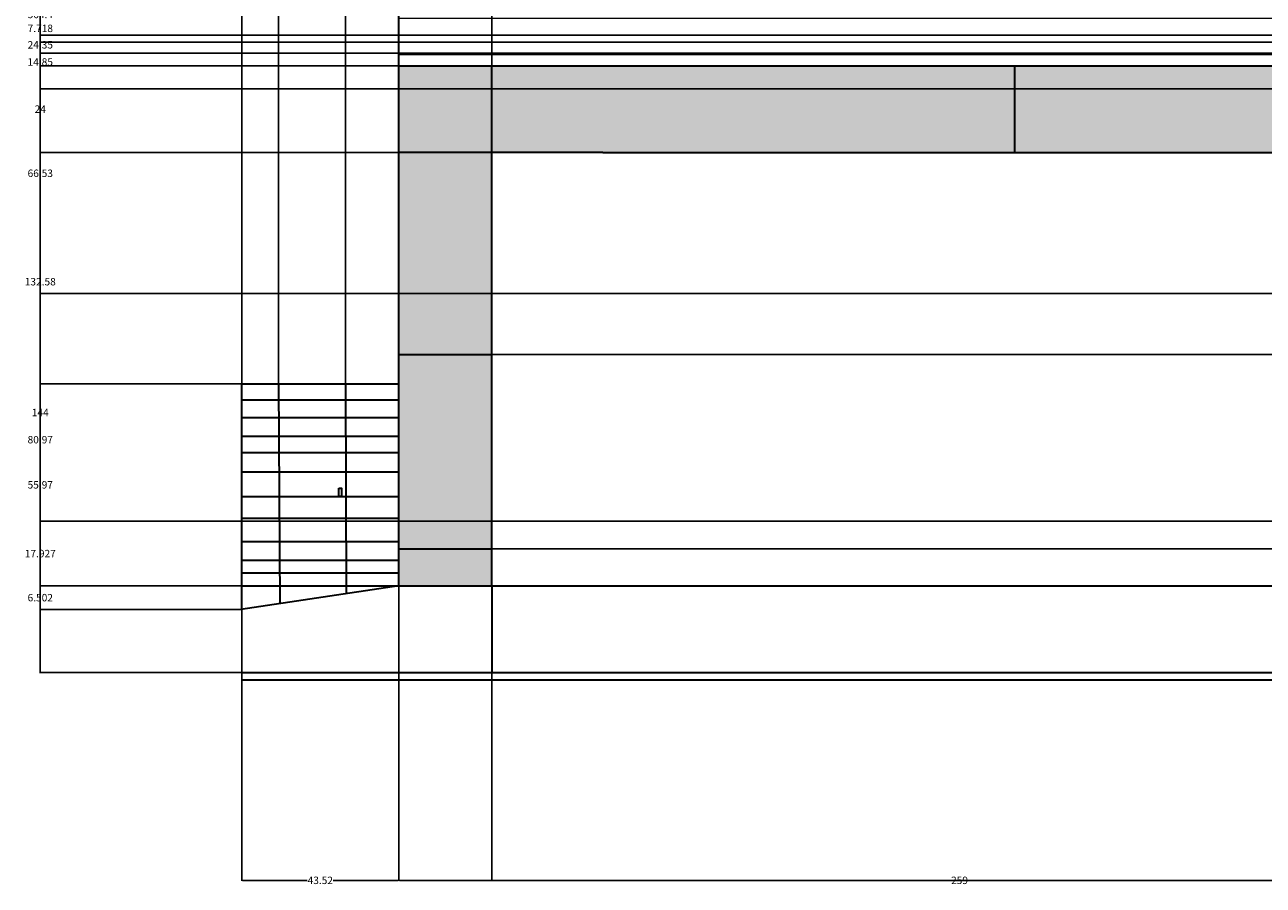
# Model space of a CAD drawing. Units: inches. Extents: x -30 to 1188, y 40 to 520.
# Tile 1 of 7: x -30 to 313, y 40 to 278. Entities that reach past the tile are written whole.
import ezdxf

# ---------------------------------------------------------------- set-up
doc = ezdxf.new("R2010")
doc.units = ezdxf.units.IN
doc.header["$MEASUREMENT"] = 0
for name, color, linetype, lineweight in [('A-ANNO-DIMS', 2, 'Continuous', 18), ('A-ELEV', 7, 'Continuous', 35), ('A-ELEV-PATT', 8, 'Continuous', 13)]:
    doc.layers.add(name, color=color, linetype=linetype, lineweight=lineweight)
doc.styles.get("Standard").update_dxf_attribs({"font": 'arial.ttf'})
doc.dimstyles.get("Standard").update_dxf_attribs({"dimtxt": 2.0625, "dimasz": 0.18, "dimexe": 0.18, "dimexo": 0.0625, "dimgap": 0.09, "dimtad": 0, "dimtih": 1, "dimtoh": 1, "dimdec": 4, "dimzin": 0, "dimdsep": 46, "dimlunit": 4, "dimtxsty": 'Standard', "dimcen": 0.09, "dimadec": 0, "dimazin": 0, "dimtfac": 1, "dimtdec": 4, "dimtofl": 0, "dimtmove": 0, "dimatfit": 3, "dimfxl": 1, "dimtolj": 1, "dimtzin": 0, "dimarcsym": 0})

# ---------------------------------------------------------------- blocks, each defined once
blk = doc.blocks.new('*D4')
at = {"layer": 'A-ANNO-DIMS', "color": 0, "lineweight": -2, "transparency": 16777216}
for p, q in [((73.66, 122.81), (73.66, 41.19)), ((1107.88, 118.31), (1107.88, 41.19)), ((73.84, 41.37), (586.5, 41.37)), ((1107.7, 41.37), (595.03, 41.37))]:
    blk.add_line(p, q, dxfattribs=at)
at = {"layer": 'A-ANNO-DIMS', "color": 0, "transparency": 16777216}
for points in [[(73.84, 41.4), (73.84, 41.34), (73.66, 41.37)], [(1107.7, 41.4), (1107.7, 41.34), (1107.88, 41.37)]]:
    blk.add_solid(points, dxfattribs=at)
at = {"layer": 'Defpoints', "color": 0, "transparency": 16777216}
for p in [(73.66, 122.87), (1107.88, 118.38), (1107.88, 41.37)]:
    blk.add_point(p, dxfattribs=at)
at = {"layer": 'A-ANNO-DIMS', "color": 0, "transparency": 16777216, "insert": (590.77, 41.37), "char_height": 2.062, "attachment_point": 5}
blk.add_mtext('\\A1;1034.2', dxfattribs=at)
blk = doc.blocks.new('*D9')
at = {"layer": 'A-ANNO-DIMS', "color": 0, "lineweight": -2, "transparency": 16777216}
for p, q in [((99.43, 98.81), (99.43, 41.19)), ((358.42, 98.81), (358.42, 41.19)), ((99.61, 41.37), (226.54, 41.37)), ((358.24, 41.37), (231.32, 41.37))]:
    blk.add_line(p, q, dxfattribs=at)
at = {"layer": 'A-ANNO-DIMS', "color": 0, "transparency": 16777216}
for points in [[(99.61, 41.4), (99.61, 41.34), (99.43, 41.37)], [(358.24, 41.4), (358.24, 41.34), (358.42, 41.37)]]:
    blk.add_solid(points, dxfattribs=at)
at = {"layer": 'Defpoints', "color": 0, "transparency": 16777216}
for p in [(99.43, 98.87), (358.42, 98.87), (358.42, 41.37)]:
    blk.add_point(p, dxfattribs=at)
at = {"layer": 'A-ANNO-DIMS', "color": 0, "transparency": 16777216, "insert": (228.93, 41.37), "char_height": 2.062, "attachment_point": 5}
blk.add_mtext('\\A1;259', dxfattribs=at)
blk = doc.blocks.new('*D10')
at = {"layer": 'A-ANNO-DIMS', "color": 0, "lineweight": -2, "transparency": 16777216}
for p, q in [((73.66, 242.93), (73.66, 518.97)), ((73.84, 518.79), (82.16, 518.79)), ((99.25, 518.79), (90.93, 518.79)), ((99.43, 242.93), (99.43, 518.97))]:
    blk.add_line(p, q, dxfattribs=at)
at = {"layer": 'A-ANNO-DIMS', "color": 0, "transparency": 16777216}
for points in [[(73.84, 518.82), (73.84, 518.76), (73.66, 518.79)], [(99.25, 518.82), (99.25, 518.76), (99.43, 518.79)]]:
    blk.add_solid(points, dxfattribs=at)
at = {"layer": 'Defpoints', "color": 0, "transparency": 16777216}
for p in [(99.43, 518.79), (73.66, 242.87), (99.43, 242.87)]:
    blk.add_point(p, dxfattribs=at)
at = {"layer": 'A-ANNO-DIMS', "color": 0, "transparency": 16777216, "insert": (86.54, 518.79), "char_height": 2.062, "attachment_point": 5}
blk.add_mtext('\\A1;25.773', dxfattribs=at)
blk = doc.blocks.new('*D11')
at = {"layer": 'A-ANNO-DIMS', "color": 0, "lineweight": -2, "transparency": 16777216}
for p, q in [((73.66, 122.81), (73.66, 41.19)), ((30.14, 98.81), (30.14, 41.19)), ((30.32, 41.37), (48.3, 41.37)), ((73.48, 41.37), (55.5, 41.37))]:
    blk.add_line(p, q, dxfattribs=at)
at = {"layer": 'A-ANNO-DIMS', "color": 0, "transparency": 16777216}
for points in [[(30.32, 41.4), (30.32, 41.34), (30.14, 41.37)], [(73.48, 41.4), (73.48, 41.34), (73.66, 41.37)]]:
    blk.add_solid(points, dxfattribs=at)
at = {"layer": 'Defpoints', "color": 0, "transparency": 16777216}
for p in [(73.66, 122.87), (30.14, 98.87), (73.66, 41.37)]:
    blk.add_point(p, dxfattribs=at)
at = {"layer": 'A-ANNO-DIMS', "color": 0, "transparency": 16777216, "insert": (51.9, 41.37), "char_height": 2.062, "attachment_point": 5}
blk.add_mtext('\\A1;43.52', dxfattribs=at)
blk = doc.blocks.new('*D18')
at = {"layer": 'A-ANNO-DIMS', "color": 0, "lineweight": -2, "transparency": 16777216}
for p, q in [((73.6, 463.29), (-25.83, 463.29)), ((-25.65, 463.11), (-25.65, 282.23)), ((-25.65, 99.05), (-25.65, 279.94)), ((30.08, 98.87), (-25.83, 98.87))]:
    blk.add_line(p, q, dxfattribs=at)
at = {"layer": 'A-ANNO-DIMS', "color": 0, "transparency": 16777216}
for points in [[(-25.68, 463.11), (-25.62, 463.11), (-25.65, 463.29)], [(-25.68, 99.05), (-25.62, 99.05), (-25.65, 98.87)]]:
    blk.add_solid(points, dxfattribs=at)
at = {"layer": 'Defpoints', "color": 0, "transparency": 16777216}
for p in [(-25.65, 463.29), (73.66, 463.29), (30.14, 98.87)]:
    blk.add_point(p, dxfattribs=at)
at = {"layer": 'A-ANNO-DIMS', "color": 0, "transparency": 16777216, "insert": (-25.65, 281.08), "char_height": 2.062, "attachment_point": 5}
blk.add_mtext('\\A1;364.4', dxfattribs=at)
blk = doc.blocks.new('*D20')
at = {"layer": 'A-ANNO-DIMS', "color": 0, "lineweight": -2, "transparency": 16777216}
for p, q in [((358.36, 242.87), (-25.83, 242.87)), ((-25.65, 242.69), (-25.65, 172)), ((-25.65, 99.05), (-25.65, 169.75)), ((358.36, 98.87), (-25.83, 98.87))]:
    blk.add_line(p, q, dxfattribs=at)
at = {"layer": 'A-ANNO-DIMS', "color": 0, "transparency": 16777216}
for points in [[(-25.68, 242.69), (-25.62, 242.69), (-25.65, 242.87)], [(-25.68, 99.05), (-25.62, 99.05), (-25.65, 98.87)]]:
    blk.add_solid(points, dxfattribs=at)
at = {"layer": 'Defpoints', "color": 0, "transparency": 16777216}
for p in [(-25.65, 242.87), (358.42, 242.87), (358.42, 98.87)]:
    blk.add_point(p, dxfattribs=at)
at = {"layer": 'A-ANNO-DIMS', "color": 0, "transparency": 16777216, "insert": (-25.65, 170.87), "char_height": 2.062, "attachment_point": 5}
blk.add_mtext('\\A1;144', dxfattribs=at)
blk = doc.blocks.new('*D29')
at = {"layer": 'A-ANNO-DIMS', "color": 0, "lineweight": -2, "transparency": 16777216}
for p, q in [((792.57, 270.37), (-25.83, 270.37)), ((-25.65, 270.19), (-25.65, 238.25)), ((-25.65, 204.02), (-25.65, 235.96)), ((792.57, 203.84), (-25.83, 203.84))]:
    blk.add_line(p, q, dxfattribs=at)
at = {"layer": 'A-ANNO-DIMS', "color": 0, "transparency": 16777216}
for points in [[(-25.68, 270.19), (-25.62, 270.19), (-25.65, 270.37)], [(-25.68, 204.02), (-25.62, 204.02), (-25.65, 203.84)]]:
    blk.add_solid(points, dxfattribs=at)
at = {"layer": 'Defpoints', "color": 0, "transparency": 16777216}
for p in [(-25.65, 270.37), (792.63, 270.37), (792.63, 203.84)]:
    blk.add_point(p, dxfattribs=at)
at = {"layer": 'A-ANNO-DIMS', "color": 0, "transparency": 16777216, "insert": (-25.65, 237.11), "char_height": 2.062, "attachment_point": 5}
blk.add_mtext('\\A1;66.53', dxfattribs=at)
blk = doc.blocks.new('*D31')
at = {"layer": 'A-ANNO-DIMS', "color": 0, "lineweight": -2, "transparency": 16777216}
for p, q in [((792.57, 203.84), (-25.83, 203.84)), ((-25.65, 203.66), (-25.65, 164.5)), ((-25.65, 123.05), (-25.65, 162.21)), ((935.84, 122.87), (-25.83, 122.87))]:
    blk.add_line(p, q, dxfattribs=at)
at = {"layer": 'A-ANNO-DIMS', "color": 0, "transparency": 16777216}
for points in [[(-25.68, 203.66), (-25.62, 203.66), (-25.65, 203.84)], [(-25.68, 123.05), (-25.62, 123.05), (-25.65, 122.87)]]:
    blk.add_solid(points, dxfattribs=at)
at = {"layer": 'Defpoints', "color": 0, "transparency": 16777216}
for p in [(792.63, 203.84), (-25.65, 122.87), (935.9, 122.87)]:
    blk.add_point(p, dxfattribs=at)
at = {"layer": 'A-ANNO-DIMS', "color": 0, "transparency": 16777216, "insert": (-25.65, 163.36), "char_height": 2.062, "attachment_point": 5}
blk.add_mtext('\\A1;80.97', dxfattribs=at)
blk = doc.blocks.new('*D33')
at = {"layer": 'A-ANNO-DIMS', "color": 0, "lineweight": -2, "transparency": 16777216}
for p, q in [((99.37, 317.88), (-25.83, 317.88)), ((-25.65, 317.7), (-25.65, 293.52)), ((-25.65, 267.05), (-25.65, 291.23)), ((73.6, 266.87), (-25.83, 266.87))]:
    blk.add_line(p, q, dxfattribs=at)
at = {"layer": 'A-ANNO-DIMS', "color": 0, "transparency": 16777216}
for points in [[(-25.68, 317.7), (-25.62, 317.7), (-25.65, 317.88)], [(-25.68, 267.05), (-25.62, 267.05), (-25.65, 266.87)]]:
    blk.add_solid(points, dxfattribs=at)
at = {"layer": 'Defpoints', "color": 0, "transparency": 16777216}
for p in [(99.43, 317.88), (-25.65, 266.87), (73.66, 266.87)]:
    blk.add_point(p, dxfattribs=at)
at = {"layer": 'A-ANNO-DIMS', "color": 0, "transparency": 16777216, "insert": (-25.65, 292.38), "char_height": 2.062, "attachment_point": 5}
blk.add_mtext('\\A1;51.01', dxfattribs=at)
blk = doc.blocks.new('*D34')
at = {"layer": 'A-ANNO-DIMS', "color": 0, "lineweight": -2, "transparency": 16777216}
for p, q in [((73.6, 266.87), (-25.83, 266.87)), ((-25.65, 266.69), (-25.65, 256)), ((-25.65, 243.05), (-25.65, 253.75)), ((73.6, 242.87), (-25.83, 242.87))]:
    blk.add_line(p, q, dxfattribs=at)
at = {"layer": 'A-ANNO-DIMS', "color": 0, "transparency": 16777216}
for points in [[(-25.68, 266.69), (-25.62, 266.69), (-25.65, 266.87)], [(-25.68, 243.05), (-25.62, 243.05), (-25.65, 242.87)]]:
    blk.add_solid(points, dxfattribs=at)
at = {"layer": 'Defpoints', "color": 0, "transparency": 16777216}
for p in [(73.66, 266.87), (-25.65, 242.87), (73.66, 242.87)]:
    blk.add_point(p, dxfattribs=at)
at = {"layer": 'A-ANNO-DIMS', "color": 0, "transparency": 16777216, "insert": (-25.65, 254.87), "char_height": 2.062, "attachment_point": 5}
blk.add_mtext('\\A1;24', dxfattribs=at)
blk = doc.blocks.new('*D35')
at = {"layer": 'A-ANNO-DIMS', "color": 0, "lineweight": -2, "transparency": 16777216}
for p, q in [((99.49, 122.87), (1183.93, 122.87)), ((1183.75, 122.69), (1183.75, 112)), ((1183.75, 99.05), (1183.75, 109.75)), ((99.49, 98.87), (1183.93, 98.87))]:
    blk.add_line(p, q, dxfattribs=at)
at = {"layer": 'A-ANNO-DIMS', "color": 0, "transparency": 16777216}
for points in [[(1183.72, 122.69), (1183.78, 122.69), (1183.75, 122.87)], [(1183.72, 99.05), (1183.78, 99.05), (1183.75, 98.87)]]:
    blk.add_solid(points, dxfattribs=at)
at = {"layer": 'Defpoints', "color": 0, "transparency": 16777216}
for p in [(99.43, 122.87), (1183.75, 122.87), (99.43, 98.87)]:
    blk.add_point(p, dxfattribs=at)
at = {"layer": 'A-ANNO-DIMS', "color": 0, "transparency": 16777216, "insert": (1183.75, 110.87), "char_height": 2.062, "attachment_point": 5}
blk.add_mtext('\\A1;24', dxfattribs=at)
blk = doc.blocks.new('*D36')
at = {"layer": 'A-ANNO-DIMS', "color": 0, "lineweight": -2, "transparency": 16777216}
for p, q in [((99.49, 133.14), (1183.93, 133.14)), ((1183.75, 132.96), (1183.75, 129.15)), ((1183.75, 123.05), (1183.75, 126.86)), ((99.49, 122.87), (1183.93, 122.87))]:
    blk.add_line(p, q, dxfattribs=at)
at = {"layer": 'A-ANNO-DIMS', "color": 0, "transparency": 16777216}
for points in [[(1183.72, 132.96), (1183.78, 132.96), (1183.75, 133.14)], [(1183.72, 123.05), (1183.78, 123.05), (1183.75, 122.87)]]:
    blk.add_solid(points, dxfattribs=at)
at = {"layer": 'Defpoints', "color": 0, "transparency": 16777216}
for p in [(99.43, 133.14), (1183.75, 133.14), (99.43, 122.87)]:
    blk.add_point(p, dxfattribs=at)
at = {"layer": 'A-ANNO-DIMS', "color": 0, "transparency": 16777216, "insert": (1183.75, 128.01), "char_height": 2.062, "attachment_point": 5}
blk.add_mtext('\\A1;10.268', dxfattribs=at)
blk = doc.blocks.new('*D37')
at = {"layer": 'A-ANNO-DIMS', "color": 0, "lineweight": -2, "transparency": 16777216}
for p, q in [((99.49, 186.93), (1183.93, 186.93)), ((1183.75, 186.75), (1183.75, 161.18)), ((1183.75, 133.32), (1183.75, 158.89)), ((99.49, 133.14), (1183.93, 133.14))]:
    blk.add_line(p, q, dxfattribs=at)
at = {"layer": 'A-ANNO-DIMS', "color": 0, "transparency": 16777216}
for points in [[(1183.72, 186.75), (1183.78, 186.75), (1183.75, 186.93)], [(1183.72, 133.32), (1183.78, 133.32), (1183.75, 133.14)]]:
    blk.add_solid(points, dxfattribs=at)
at = {"layer": 'Defpoints', "color": 0, "transparency": 16777216}
for p in [(99.43, 186.93), (1183.75, 186.93), (99.43, 133.14)]:
    blk.add_point(p, dxfattribs=at)
at = {"layer": 'A-ANNO-DIMS', "color": 0, "transparency": 16777216, "insert": (1183.75, 160.03), "char_height": 2.062, "attachment_point": 5}
blk.add_mtext('\\A1;53.79', dxfattribs=at)
blk = doc.blocks.new('*D38')
at = {"layer": 'A-ANNO-DIMS', "color": 0, "lineweight": -2, "transparency": 16777216}
for p, q in [((99.49, 242.87), (1183.93, 242.87)), ((1183.75, 242.69), (1183.75, 216.04)), ((1183.75, 187.11), (1183.75, 213.76)), ((99.49, 186.93), (1183.93, 186.93))]:
    blk.add_line(p, q, dxfattribs=at)
at = {"layer": 'A-ANNO-DIMS', "color": 0, "transparency": 16777216}
for points in [[(1183.72, 242.69), (1183.78, 242.69), (1183.75, 242.87)], [(1183.72, 187.11), (1183.78, 187.11), (1183.75, 186.93)]]:
    blk.add_solid(points, dxfattribs=at)
at = {"layer": 'Defpoints', "color": 0, "transparency": 16777216}
for p in [(99.43, 242.87), (1183.75, 242.87), (99.43, 186.93)]:
    blk.add_point(p, dxfattribs=at)
at = {"layer": 'A-ANNO-DIMS', "color": 0, "transparency": 16777216, "insert": (1183.75, 214.9), "char_height": 2.062, "attachment_point": 5}
blk.add_mtext('\\A1;55.94', dxfattribs=at)
blk = doc.blocks.new('*D44')
at = {"layer": 'A-ANNO-DIMS', "color": 0, "lineweight": -2, "transparency": 16777216}
for p, q in [((980.66, 275.34), (-25.83, 275.34)), ((-25.65, 275.16), (-25.65, 269.06)), ((-25.65, 260.67), (-25.65, 266.77)), ((980.66, 260.49), (-25.83, 260.49))]:
    blk.add_line(p, q, dxfattribs=at)
at = {"layer": 'A-ANNO-DIMS', "color": 0, "transparency": 16777216}
for points in [[(-25.68, 275.16), (-25.62, 275.16), (-25.65, 275.34)], [(-25.68, 260.67), (-25.62, 260.67), (-25.65, 260.49)]]:
    blk.add_solid(points, dxfattribs=at)
at = {"layer": 'Defpoints', "color": 0, "transparency": 16777216}
for p in [(-25.65, 275.34), (980.73, 275.34), (980.73, 260.49)]:
    blk.add_point(p, dxfattribs=at)
at = {"layer": 'A-ANNO-DIMS', "color": 0, "transparency": 16777216, "insert": (-25.65, 267.92), "char_height": 2.062, "attachment_point": 5}
blk.add_mtext('\\A1;14.85', dxfattribs=at)
blk = doc.blocks.new('*D45')
at = {"layer": 'A-ANNO-DIMS', "color": 0, "lineweight": -2, "transparency": 16777216}
for p, q in [((945.03, 284.84), (-25.83, 284.84)), ((-25.65, 284.66), (-25.65, 273.81)), ((-25.65, 260.67), (-25.65, 271.52)), ((935.84, 260.49), (-25.83, 260.49))]:
    blk.add_line(p, q, dxfattribs=at)
at = {"layer": 'A-ANNO-DIMS', "color": 0, "transparency": 16777216}
for points in [[(-25.68, 284.66), (-25.62, 284.66), (-25.65, 284.84)], [(-25.68, 260.67), (-25.62, 260.67), (-25.65, 260.49)]]:
    blk.add_solid(points, dxfattribs=at)
at = {"layer": 'Defpoints', "color": 0, "transparency": 16777216}
for p in [(945.1, 284.84), (-25.65, 260.49), (935.9, 260.49)]:
    blk.add_point(p, dxfattribs=at)
at = {"layer": 'A-ANNO-DIMS', "color": 0, "transparency": 16777216, "insert": (-25.65, 272.67), "char_height": 2.062, "attachment_point": 5}
blk.add_mtext('\\A1;24.35', dxfattribs=at)
blk = doc.blocks.new('*D50')
at = {"layer": 'A-ANNO-DIMS', "color": 0, "lineweight": -2, "transparency": 16777216}
for p, q in [((73.6, 122.87), (-25.83, 122.87)), ((-25.65, 122.69), (-25.65, 120.76)), ((-25.65, 116.55), (-25.65, 118.48)), ((30.08, 116.37), (-25.83, 116.37))]:
    blk.add_line(p, q, dxfattribs=at)
at = {"layer": 'A-ANNO-DIMS', "color": 0, "transparency": 16777216}
for points in [[(-25.68, 122.69), (-25.62, 122.69), (-25.65, 122.87)], [(-25.68, 116.55), (-25.62, 116.55), (-25.65, 116.37)]]:
    blk.add_solid(points, dxfattribs=at)
at = {"layer": 'Defpoints', "color": 0, "transparency": 16777216}
for p in [(-25.65, 122.87), (73.66, 122.87), (30.14, 116.37)]:
    blk.add_point(p, dxfattribs=at)
at = {"layer": 'A-ANNO-DIMS', "color": 0, "transparency": 16777216, "insert": (-25.65, 119.62), "char_height": 2.062, "attachment_point": 5}
blk.add_mtext('\\A1;6.502', dxfattribs=at)
blk = doc.blocks.new('*D51')
at = {"layer": 'A-ANNO-DIMS', "color": 0, "lineweight": -2, "transparency": 16777216}
for p, q in [((30.08, 178.84), (-25.83, 178.84)), ((-25.65, 178.66), (-25.65, 152)), ((-25.65, 123.05), (-25.65, 149.71)), ((73.6, 122.87), (-25.83, 122.87))]:
    blk.add_line(p, q, dxfattribs=at)
at = {"layer": 'A-ANNO-DIMS', "color": 0, "transparency": 16777216}
for points in [[(-25.68, 178.66), (-25.62, 178.66), (-25.65, 178.84)], [(-25.68, 123.05), (-25.62, 123.05), (-25.65, 122.87)]]:
    blk.add_solid(points, dxfattribs=at)
at = {"layer": 'Defpoints', "color": 0, "transparency": 16777216}
for p in [(-25.65, 178.84), (30.14, 178.84), (73.66, 122.87)]:
    blk.add_point(p, dxfattribs=at)
at = {"layer": 'A-ANNO-DIMS', "color": 0, "transparency": 16777216, "insert": (-25.65, 150.86), "char_height": 2.062, "attachment_point": 5}
blk.add_mtext('\\A1;55.97', dxfattribs=at)
blk = doc.blocks.new('*D52')
at = {"layer": 'A-ANNO-DIMS', "color": 0, "lineweight": -2, "transparency": 16777216}
for p, q in [((30.14, 178.91), (30.14, 518.97)), ((30.32, 518.79), (30.95, 518.79)), ((40.14, 518.79), (39.5, 518.79)), ((40.32, 178.91), (40.32, 518.97))]:
    blk.add_line(p, q, dxfattribs=at)
at = {"layer": 'A-ANNO-DIMS', "color": 0, "transparency": 16777216}
for points in [[(30.32, 518.82), (30.32, 518.76), (30.14, 518.79)], [(40.14, 518.82), (40.14, 518.76), (40.32, 518.79)]]:
    blk.add_solid(points, dxfattribs=at)
at = {"layer": 'Defpoints', "color": 0, "transparency": 16777216}
for p in [(40.32, 518.79), (30.14, 178.84), (40.32, 178.84)]:
    blk.add_point(p, dxfattribs=at)
at = {"layer": 'A-ANNO-DIMS', "color": 0, "transparency": 16777216, "insert": (35.23, 518.79), "char_height": 2.062, "attachment_point": 5}
blk.add_mtext('\\A1;10.177', dxfattribs=at)
blk = doc.blocks.new('*D53')
at = {"layer": 'A-ANNO-DIMS', "color": 0, "lineweight": -2, "transparency": 16777216}
for p, q in [((40.32, 178.91), (40.32, 518.97)), ((40.5, 518.79), (45.32, 518.79)), ((58.68, 518.79), (53.86, 518.79)), ((58.86, 178.91), (58.86, 518.97))]:
    blk.add_line(p, q, dxfattribs=at)
at = {"layer": 'A-ANNO-DIMS', "color": 0, "transparency": 16777216}
for points in [[(40.5, 518.82), (40.5, 518.76), (40.32, 518.79)], [(58.68, 518.82), (58.68, 518.76), (58.86, 518.79)]]:
    blk.add_solid(points, dxfattribs=at)
at = {"layer": 'Defpoints', "color": 0, "transparency": 16777216}
for p in [(58.86, 518.79), (40.32, 178.84), (58.86, 178.84)]:
    blk.add_point(p, dxfattribs=at)
at = {"layer": 'A-ANNO-DIMS', "color": 0, "transparency": 16777216, "insert": (49.59, 518.79), "char_height": 2.062, "attachment_point": 5}
blk.add_mtext('\\A1;18.544', dxfattribs=at)
blk = doc.blocks.new('*D54')
at = {"layer": 'A-ANNO-DIMS', "color": 0, "lineweight": -2, "transparency": 16777216}
for p, q in [((58.86, 178.91), (58.86, 518.97)), ((59.04, 518.79), (61.98, 518.79)), ((73.48, 518.79), (70.54, 518.79)), ((73.66, 178.91), (73.66, 518.97))]:
    blk.add_line(p, q, dxfattribs=at)
at = {"layer": 'A-ANNO-DIMS', "color": 0, "transparency": 16777216}
for points in [[(59.04, 518.82), (59.04, 518.76), (58.86, 518.79)], [(73.48, 518.82), (73.48, 518.76), (73.66, 518.79)]]:
    blk.add_solid(points, dxfattribs=at)
at = {"layer": 'Defpoints', "color": 0, "transparency": 16777216}
for p in [(73.66, 518.79), (58.86, 178.84), (73.66, 178.84)]:
    blk.add_point(p, dxfattribs=at)
at = {"layer": 'A-ANNO-DIMS', "color": 0, "transparency": 16777216, "insert": (66.26, 518.79), "char_height": 2.062, "attachment_point": 5}
blk.add_mtext('\\A1;14.798', dxfattribs=at)
blk = doc.blocks.new('*D55')
at = {"layer": 'A-ANNO-DIMS', "color": 0, "lineweight": -2, "transparency": 16777216}
for p, q in [((466.76, 140.8), (-25.83, 140.8)), ((-25.65, 140.62), (-25.65, 132.98)), ((-25.65, 123.05), (-25.65, 130.69)), ((466.93, 122.87), (-25.83, 122.87))]:
    blk.add_line(p, q, dxfattribs=at)
at = {"layer": 'A-ANNO-DIMS', "color": 0, "transparency": 16777216}
for points in [[(-25.68, 140.62), (-25.62, 140.62), (-25.65, 140.8)], [(-25.68, 123.05), (-25.62, 123.05), (-25.65, 122.87)]]:
    blk.add_solid(points, dxfattribs=at)
at = {"layer": 'Defpoints', "color": 0, "transparency": 16777216}
for p in [(-25.65, 140.8), (466.83, 140.8), (467, 122.87)]:
    blk.add_point(p, dxfattribs=at)
at = {"layer": 'A-ANNO-DIMS', "color": 0, "transparency": 16777216, "insert": (-25.65, 131.83), "char_height": 2.062, "attachment_point": 5}
blk.add_mtext('\\A1;17.927', dxfattribs=at)
blk = doc.blocks.new('*D56')
at = {"layer": 'A-ANNO-DIMS', "color": 0, "lineweight": -2, "transparency": 16777216}
for p, q in [((466.76, 273.38), (-25.83, 273.38)), ((-25.65, 273.2), (-25.65, 208.23)), ((-25.65, 140.98), (-25.65, 205.94)), ((466.76, 140.8), (-25.83, 140.8))]:
    blk.add_line(p, q, dxfattribs=at)
at = {"layer": 'A-ANNO-DIMS', "color": 0, "transparency": 16777216}
for points in [[(-25.68, 273.2), (-25.62, 273.2), (-25.65, 273.38)], [(-25.68, 140.98), (-25.62, 140.98), (-25.65, 140.8)]]:
    blk.add_solid(points, dxfattribs=at)
at = {"layer": 'Defpoints', "color": 0, "transparency": 16777216}
for p in [(-25.65, 273.38), (466.83, 273.38), (466.83, 140.8)]:
    blk.add_point(p, dxfattribs=at)
at = {"layer": 'A-ANNO-DIMS', "color": 0, "transparency": 16777216, "insert": (-25.65, 207.09), "char_height": 2.062, "attachment_point": 5}
blk.add_mtext('\\A1;132.58', dxfattribs=at)
blk = doc.blocks.new('*D57')
at = {"layer": 'A-ANNO-DIMS', "color": 0, "lineweight": -2, "transparency": 16777216}
for p, q in [((466.93, 281.09), (-25.83, 281.09)), ((-25.65, 280.91), (-25.65, 278.38)), ((-25.65, 273.56), (-25.65, 276.09)), ((466.76, 273.38), (-25.83, 273.38))]:
    blk.add_line(p, q, dxfattribs=at)
at = {"layer": 'A-ANNO-DIMS', "color": 0, "transparency": 16777216}
for points in [[(-25.68, 280.91), (-25.62, 280.91), (-25.65, 281.09)], [(-25.68, 273.56), (-25.62, 273.56), (-25.65, 273.38)]]:
    blk.add_solid(points, dxfattribs=at)
at = {"layer": 'Defpoints', "color": 0, "transparency": 16777216}
for p in [(-25.65, 281.09), (467, 281.09), (466.83, 273.38)]:
    blk.add_point(p, dxfattribs=at)
at = {"layer": 'A-ANNO-DIMS', "color": 0, "transparency": 16777216, "insert": (-25.65, 277.23), "char_height": 2.062, "attachment_point": 5}
blk.add_mtext('\\A1;7.718', dxfattribs=at)
blk = doc.blocks.new('*D74')
at = {"layer": 'A-ANNO-DIMS', "color": 0, "lineweight": -2, "transparency": 16777216}
for p, q in [((30.14, 98.93), (30.14, 518.97)), ((30.32, 518.79), (574.32, 518.79)), ((1128.07, 518.79), (584.07, 518.79)), ((1128.25, 117.62), (1128.25, 518.97))]:
    blk.add_line(p, q, dxfattribs=at)
at = {"layer": 'A-ANNO-DIMS', "color": 0, "transparency": 16777216}
for points in [[(30.32, 518.82), (30.32, 518.76), (30.14, 518.79)], [(1128.07, 518.82), (1128.07, 518.76), (1128.25, 518.79)]]:
    blk.add_solid(points, dxfattribs=at)
at = {"layer": 'Defpoints', "color": 0, "transparency": 16777216}
for p in [(1128.25, 518.79), (1128.25, 117.56), (30.14, 98.87)]:
    blk.add_point(p, dxfattribs=at)
at = {"layer": 'A-ANNO-DIMS', "color": 0, "transparency": 16777216, "insert": (579.19, 518.79), "char_height": 2.0625, "attachment_point": 5}
blk.add_mtext('\\A1;1098.11', dxfattribs=at)

msp = doc.modelspace()

# ---------------------------------------------------------------- hatches: boundary and pattern name
at = {"layer": 'A-ELEV-PATT'}
h = msp.add_hatch(dxfattribs=at)
h.set_pattern_fill('ANSI31', color=256, scale=80, angle=135)
h.paths.add_polyline_path([(935.904, 461.2934), (655.0318, 461.2934), (655.0318, 408.0708), (655.0318, 380.8615), (798.3036, 380.8615), (798.3036, 314.3348), (655.0318, 314.3348), (655.0318, 303.0545), (655.0318, 122.8714), (744.4225, 122.8714), (796.5546, 122.8714), (935.904, 122.8714), (935.904, 203.8438), (792.6322, 203.8438), (792.6322, 270.3705), (935.904, 270.3705), (935.904, 372.8284)])
h.paths.add_polyline_path([(466.9951, 434.8714), (466.9951, 461.2934), (73.6582, 461.2934), (73.6582, 434.8714), (73.6582, 410.8714), (73.6582, 266.8714), (382.4247, 266.8714), (466.9951, 266.8714)])
h.paths.add_polyline_path([(422.6392, 390.3227), (422.6392, 317.8826), (99.4312, 317.8826), (99.4312, 390.3227)], flags=16)
h.paths.add_polyline_path([(416.8376, 385.9009), (416.8376, 322.3026), (332.2885, 322.3026), (332.2885, 385.9009)], flags=0)
h.paths.add_polyline_path([(187.4151, 386.0591), (187.4151, 322.4608), (102.866, 322.4608), (102.866, 386.0591)], flags=0)
h = msp.add_hatch(color=256, dxfattribs=at)
h.dxf.hatch_style = 1
h.paths.add_polyline_path([(99.4312, 186.9265), (73.6582, 186.9265), (73.6582, 133.1393), (99.4312, 133.1393)])
h.paths.add_polyline_path([(99.4312, 242.8714), (73.6582, 242.8714), (73.6582, 186.9265), (99.4312, 186.9265)])
h.paths.add_polyline_path([(99.4312, 266.8714), (73.6582, 266.8714), (73.6582, 242.8714), (99.4312, 242.8714)])
h.paths.add_polyline_path([(244.2768, 266.8714), (99.4312, 266.8714), (99.4312, 242.8714), (130.129, 242.8714), (244.2768, 242.8714)])
h.paths.add_polyline_path([(358.4247, 266.8714), (244.2768, 266.8714), (244.2768, 242.8714), (358.4247, 242.8714)])
h.paths.add_polyline_path([(466.8255, 266.8714), (382.4247, 266.8714), (358.4247, 266.8714), (358.4247, 242.8714), (382.4247, 242.8714), (466.8255, 242.8714)])
h.paths.add_polyline_path([(466.8255, 242.8714), (382.4247, 242.8714), (358.4247, 242.8714), (358.4247, 186.9265), (382.4247, 186.9265), (466.8255, 186.9265)])
h.paths.add_polyline_path([(466.8255, 186.9265), (382.4247, 186.9265), (358.4247, 186.9265), (358.4247, 133.1393), (382.4247, 133.1393), (466.9951, 133.1393), (466.9951, 140.7981), (466.8255, 140.7981)])
h.paths.add_polyline_path([(521.0073, 303.0545), (466.9951, 303.0545), (466.9951, 281.0934), (521.0073, 281.0934)])
h.paths.add_polyline_path([(588.0971, 303.0545), (521.0073, 303.0545), (521.0073, 281.0934), (588.0971, 281.0934)])
h.paths.add_polyline_path([(655.0318, 303.0545), (588.0971, 303.0545), (588.0971, 281.0934), (655.0318, 281.0934)])
h.paths.add_polyline_path([(655.0318, 408.0708), (655.0318, 418.5083), (588.0971, 418.5083), (588.0971, 390.7733), (655.0318, 390.7733)])
h.paths.add_polyline_path([(588.0971, 418.5083), (521.0073, 418.5083), (521.0073, 390.7733), (588.0971, 390.7733)])
h.paths.add_polyline_path([(521.0073, 418.5083), (466.9951, 418.5083), (466.9951, 390.7733), (521.0073, 390.7733)])
h = msp.add_hatch(color=256, dxfattribs=at)
h.dxf.hatch_style = 1
h.paths.add_polyline_path([(99.4312, 133.1393), (73.6582, 133.1393), (73.6582, 122.8714), (99.4312, 122.8714)])
h.paths.add_polyline_path([(466.9951, 133.1393), (382.4247, 133.1393), (358.4247, 133.1393), (358.4247, 122.8714), (435.3376, 122.8714), (466.9951, 122.8714)])

# ---------------------------------------------------------------- linework, layer by layer
at = {"layer": 'A-ELEV'}
for p, q in [((73.6582, 266.8714), (73.6582, 410.8714)), ((73.6582, 122.8714), (73.6582, 266.8714)), ((73.6582, 266.8714), (382.4247, 266.8714)), ((99.4312, 242.8714), (99.4312, 266.8714)), ((244.2768, 242.8714), (244.2768, 266.8714)), ((99.4312, 242.8714), (73.6582, 242.8714)), ((99.4312, 122.8714), (99.4312, 242.8714)), ((130.129, 242.8714), (99.4312, 242.8714)), ((130.129, 242.8714), (358.4247, 242.8714)), ((73.6582, 186.9265), (99.4312, 186.9265)), ((30.1395, 116.3695), (30.1395, 178.8431)), ((30.1395, 178.8431), (73.6582, 178.8431)), ((40.3164, 178.8431), (40.6798, 117.9443)), ((58.8603, 178.8431), (59.0872, 120.6945)), ((30.0719, 174.3771), (73.6582, 174.3771)), ((30.0719, 169.5024), (73.6582, 169.5024)), ((30.0719, 164.3131), (73.6582, 164.3131)), ((30.0719, 159.8158), (73.6582, 159.8158)), ((30.0719, 154.4536), (73.6582, 154.4536)), ((30.0719, 147.6063), (73.6582, 147.6063)), ((30.0719, 141.6089), (73.6582, 141.6089)), ((30.0719, 135.1338), (73.6582, 135.1338)), ((73.6582, 133.1393), (99.4312, 133.1393)), ((30.0719, 130.034), (73.6582, 130.034)), ((30.0719, 126.4981), (73.6582, 126.4981)), ((73.6582, 122.8714), (29.8516, 116.3265)), ((30.1395, 122.8714), (435.3376, 122.8714)), ((99.4312, 122.8714), (99.4312, 98.8714)), ((30.1395, 98.8714), (435.3376, 98.8714)), ((30.1395, 96.8714), (435.3376, 96.8714))]:
    msp.add_line(p, q, dxfattribs=at)
msp.add_lwpolyline([(57.0504, 149.9429), (57.7579, 149.9429), (57.7579, 147.6063), (57.0504, 147.6063)], close=True, dxfattribs=at)

# ---------------------------------------------------------------- dimensions: what is measured, and where the dimension line sits
at = {"layer": 'A-ANNO-DIMS'}
for base, p1, p2, override, picture, middle in [((40.3164, 518.7934), (30.1395, 178.8431), (40.3164, 178.8431), {"dimdec": 3, "dimlfac": 1, "dimrnd": 0, "dimzin": 0, "dimdsep": 46, "dimlunit": 2}, '*D52', (35.228, 518.7934)), ((1128.2474, 518.7934), (30.1395, 98.8714), (1128.2474, 117.5588), {"dimdec": 2, "dimlfac": 1, "dimrnd": 0, "dimzin": 0, "dimdsep": 46, "dimlunit": 2}, '*D74', (579.1935, 518.7934)), ((58.8603, 518.7934), (40.3164, 178.8431), (58.8603, 178.8431), {"dimdec": 3, "dimlfac": 1, "dimrnd": 0, "dimzin": 0, "dimdsep": 46, "dimlunit": 2}, '*D53', (49.5883, 518.7934)), ((73.6582, 518.7934), (58.8603, 178.8431), (73.6582, 178.8431), {"dimdec": 3, "dimlfac": 1, "dimrnd": 0, "dimzin": 0, "dimdsep": 46, "dimlunit": 2}, '*D54', (66.2592, 518.7934)), ((99.4312, 518.7934), (73.6582, 242.8714), (99.4312, 242.8714), {"dimdec": 3, "dimlfac": 1, "dimrnd": 0, "dimzin": 0, "dimdsep": 46, "dimlunit": 2}, '*D10', (86.5447, 518.7934)), ((73.6582, 41.3714), (30.1395, 98.8714), (73.6582, 122.8714), {"dimdec": 2, "dimlfac": 1, "dimrnd": 0, "dimzin": 0, "dimdsep": 46, "dimlunit": 2}, '*D11', (51.8989, 41.3714)), ((1107.8751, 41.3714), (73.6582, 122.8714), (1107.8751, 118.3767), {"dimdec": 1, "dimlfac": 1, "dimrnd": 0, "dimzin": 0, "dimdsep": 46, "dimlunit": 2}, '*D4', (590.7666, 41.3714)), ((358.4247, 41.3714), (99.4312, 98.8714), (358.4247, 98.8714), {"dimdec": 0, "dimlfac": 1, "dimrnd": 0, "dimzin": 0, "dimdsep": 46, "dimlunit": 2}, '*D9', (228.9279, 41.3714))]:
    dim = msp.add_linear_dim(base=base, p1=p1, p2=p2, dimstyle='Standard', override=override, dxfattribs=at)
    dim.commit()
    dim.dimension.update_dxf_attribs({"geometry": picture, "text_midpoint": middle})
for base, p1, p2, override, picture, middle in [((-25.6484, 463.2934), (30.1395, 98.8714), (73.6582, 463.2934), {"dimdec": 1, "dimlfac": 1, "dimrnd": 0, "dimzin": 0, "dimdsep": 46, "dimlunit": 2}, '*D18', (-25.6484, 281.0824)), ((-25.6484, 266.8714), (99.4312, 317.8826), (73.6582, 266.8714), {"dimdec": 2, "dimlfac": 1, "dimrnd": 0, "dimzin": 0, "dimdsep": 46, "dimlunit": 2}, '*D33', (-25.6484, 292.377)), ((-25.6484, 260.4906), (945.0964, 284.8425), (935.904, 260.4906), {"dimdec": 2, "dimlfac": 1, "dimrnd": 0, "dimzin": 0, "dimdsep": 46, "dimlunit": 2}, '*D45', (-25.6484, 272.6666)), ((-25.6484, 281.0934), (466.8255, 273.3754), (466.9951, 281.0934), {"dimdec": 3, "dimlfac": 1, "dimrnd": 0, "dimzin": 0, "dimdsep": 46, "dimlunit": 2}, '*D57', (-25.6484, 277.2344)), ((-25.6484, 275.3408), (980.7252, 260.4906), (980.7252, 275.3408), {"dimdec": 2, "dimlfac": 1, "dimrnd": 0, "dimzin": 0, "dimdsep": 46, "dimlunit": 2}, '*D44', (-25.6484, 267.9157)), ((-25.6484, 273.3754), (466.8255, 140.7981), (466.8255, 273.3754), {"dimdec": 2, "dimlfac": 1, "dimrnd": 0, "dimzin": 0, "dimdsep": 46, "dimlunit": 2}, '*D56', (-25.6484, 207.0867)), ((-25.6484, 270.3705), (792.6322, 203.8438), (792.6322, 270.3705), {"dimdec": 2, "dimlfac": 1, "dimrnd": 0, "dimzin": 0, "dimdsep": 46, "dimlunit": 2}, '*D29', (-25.6484, 237.1071)), ((-25.6484, 242.8714), (73.6582, 266.8714), (73.6582, 242.8714), {"dimdec": 0, "dimlfac": 1, "dimrnd": 0, "dimzin": 0, "dimdsep": 46, "dimlunit": 2}, '*D34', (-25.6484, 254.8714)), ((-25.6484, 242.8714), (358.4247, 98.8714), (358.4247, 242.8714), {"dimdec": 0, "dimlfac": 1, "dimrnd": 0, "dimzin": 0, "dimdsep": 46, "dimlunit": 2}, '*D20', (-25.6484, 170.8714)), ((1183.7474, 242.8714), (99.4312, 186.9265), (99.4312, 242.8714), {"dimdec": 2, "dimlfac": 1, "dimrnd": 0, "dimzin": 0, "dimdsep": 46, "dimlunit": 2}, '*D38', (1183.7474, 214.899)), ((-25.6484, 122.8714), (792.6322, 203.8438), (935.904, 122.8714), {"dimdec": 2, "dimlfac": 1, "dimrnd": 0, "dimzin": 0, "dimdsep": 46, "dimlunit": 2}, '*D31', (-25.6484, 163.3576)), ((1183.7474, 186.9265), (99.4312, 133.1393), (99.4312, 186.9265), {"dimdec": 2, "dimlfac": 1, "dimrnd": 0, "dimzin": 0, "dimdsep": 46, "dimlunit": 2}, '*D37', (1183.7474, 160.0329)), ((-25.6484, 178.8431), (73.6582, 122.8714), (30.1395, 178.8431), {"dimdec": 2, "dimlfac": 1, "dimrnd": 0, "dimzin": 0, "dimdsep": 46, "dimlunit": 2}, '*D51', (-25.6484, 150.8573)), ((-25.6484, 140.7981), (466.9951, 122.8714), (466.8255, 140.7981), {"dimdec": 3, "dimlfac": 1, "dimrnd": 0, "dimzin": 0, "dimdsep": 46, "dimlunit": 2}, '*D55', (-25.6484, 131.8348)), ((1183.7474, 133.1393), (99.4312, 122.8714), (99.4312, 133.1393), {"dimdec": 3, "dimlfac": 1, "dimrnd": 0, "dimzin": 0, "dimdsep": 46, "dimlunit": 2}, '*D36', (1183.7474, 128.0054)), ((-25.6484, 122.8714), (30.1395, 116.3695), (73.6582, 122.8714), {"dimdec": 3, "dimlfac": 1, "dimrnd": 0, "dimzin": 0, "dimdsep": 46, "dimlunit": 2}, '*D50', (-25.6484, 119.6205)), ((1183.7474, 122.8714), (99.4312, 98.8714), (99.4312, 122.8714), {"dimdec": 0, "dimlfac": 1, "dimrnd": 0, "dimzin": 0, "dimdsep": 46, "dimlunit": 2}, '*D35', (1183.7474, 110.8714))]:
    dim = msp.add_linear_dim(base=base, p1=p1, p2=p2, angle=90, dimstyle='Standard', override=override, dxfattribs=at)
    dim.commit()
    dim.dimension.update_dxf_attribs({"geometry": picture, "text_midpoint": middle})

doc.saveas('drawing.dxf')
